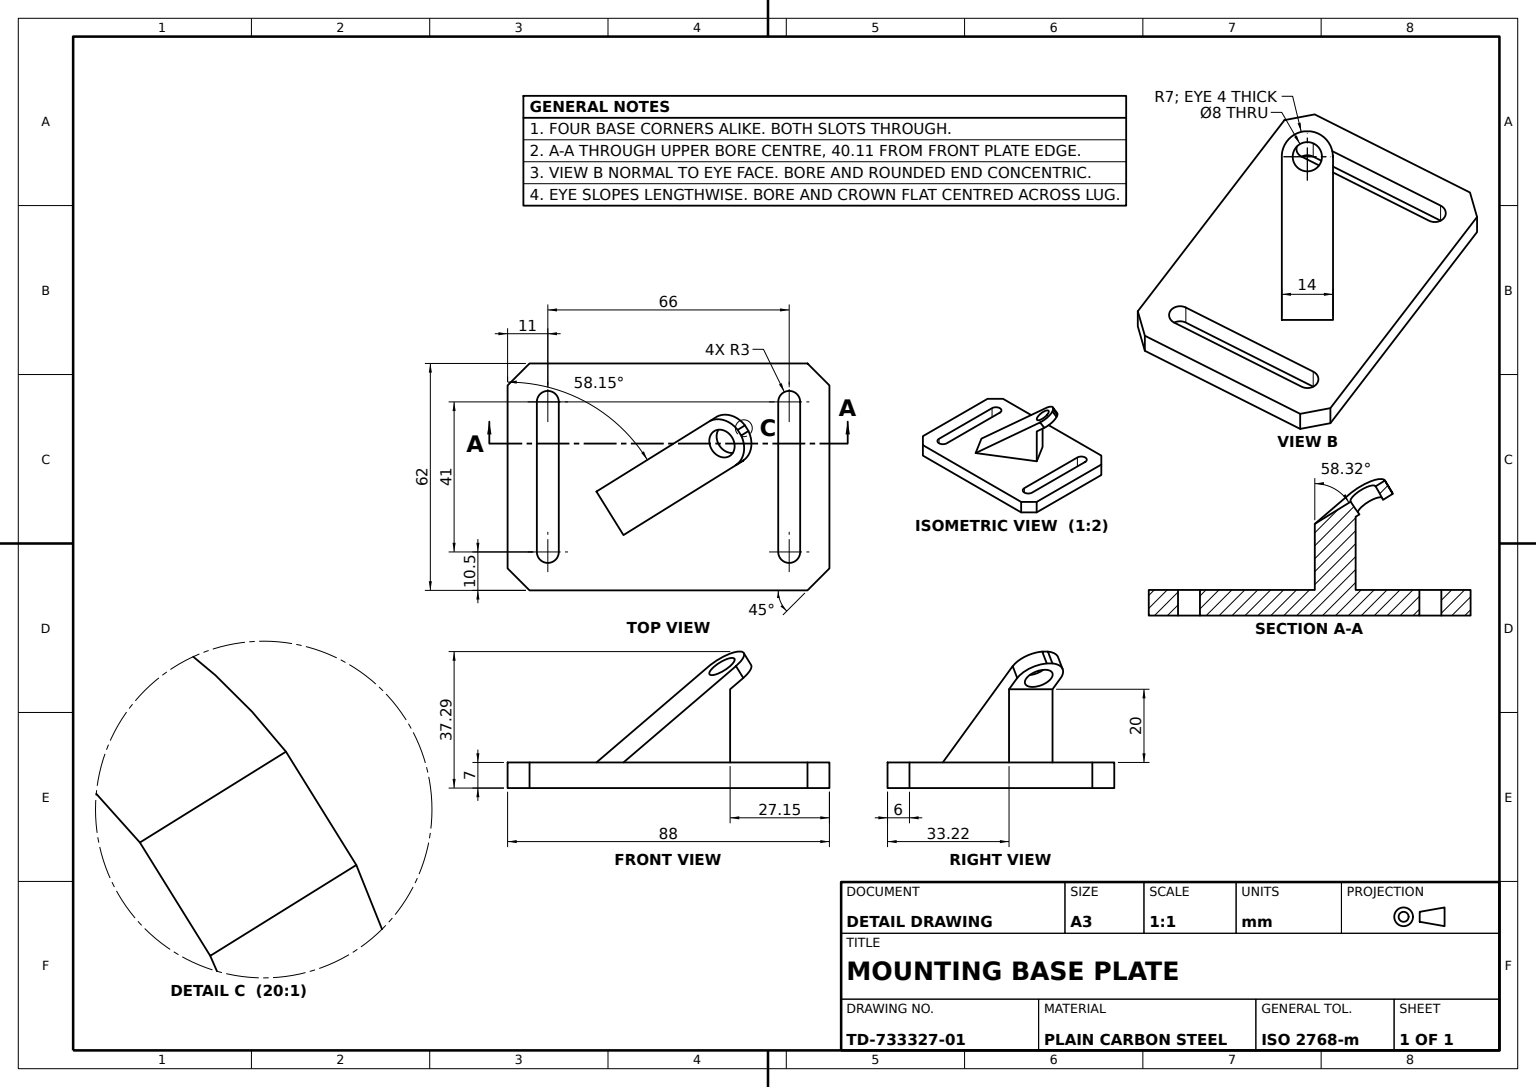
SolidWorks part; units mm, degrees
material "Plain Carbon Steel"
ref_plane "Front Plane" through (0, 0, 0) normal (0, 0, 1) x (1, 0, 0)
ref_plane "Top Plane" through (0, 0, 0) normal (0, 1, 0) x (1, 0, 0)
ref_plane "Right Plane" through (0, 0, 0) normal (1, 0, 0) x (0, 0, -1)
sketch "Base Plate Profile" plane through (0, 0, 0) normal (0, 1, 0) x (1, 0, 0)
  line L0 (-33, 20.5) -> (-33, -20.5) construction
  line L1 (-44, -31) -> (44, -31)
  line L2 (-44, -31) -> (-44, 31)
  line L3 (-44, 31) -> (44, 31)
  line L4 (44, -31) -> (44, 31)
  line L5 (-30, 20.5) -> (-30, -20.5)
  line L6 (-36, 20.5) -> (-36, -20.5)
  line L7 (33, 20.5) -> (33, -20.5) construction
  line L8 (36, 20.5) -> (36, -20.5)
  line L9 (30, 20.5) -> (30, -20.5)
  arc A0 (-30, 20.5) -> (-36, 20.5) centre (-33, 20.5) ccw
  arc A1 (-36, -20.5) -> (-30, -20.5) centre (-33, -20.5) ccw
  arc A2 (36, 20.5) -> (30, 20.5) centre (33, 20.5) ccw
  arc A3 (30, -20.5) -> (36, -20.5) centre (33, -20.5) ccw
  point P0 (0, 0)
  point P8 (-33, 0)
  point P13 (33, 0)
  dimension "D1" = 88
  dimension "D2" = 62
  dimension "D3" = 6
  dimension "D4" = 6
  dimension "D5" = 8
  dimension "D6" = 8
  dimension "D7" = 44
  dimension "D8" = 10.5
  dimension "D9" = 31
  dimension "D10" = 10.5
  dimension "D11" = 41
  dimension "D12" = 41
extrude "Base Plate 88x62x7" add sketch "Base Plate Profile" along normal blind 7
chamfer "Plate Edge Chamfer 6mm" distance 6 angle 45 4 edges at (-44, 3.5, -31) (44, 3.5, -31) (44, 3.5, 31) (-44, 3.5, 31)
sketch "Lug Profile" plane through (0, 7, 0) normal (0, 1, 0) x (1, 0, 0)
  line L0 (-19.705, -4.0002) -> (-12.3174, -15.8924)
  line L1 (-12.3174, -15.8924) -> (49.797, 22.6938)
  line L2 (49.797, 22.6938) -> (42.4094, 34.5859)
  line L3 (-55.7736, -34.6473) -> (54.8921, 34.0997) construction
  line L4 (42.4094, 34.5859) -> (-19.705, -4.0002)
  line L5 (-44, 25) -> (-44, -25) construction
  line L6 (38, 31) -> (-38, 31) construction
  dimension "D1" = 14
  dimension "D2" = 7
  dimension "D3" = 24.295
  dimension "D4" = 86.4094
  dimension "D5" = 31.6826
  dimension "D6" = 3.5859
extrude "Lifting Lug" add sketch "Lug Profile" along normal blind 87
sketch "Lug Taper Cut Profile" plane through (3.6938, 0, 5.9461) normal (0.5277, 0, 0.8494) x (0.8494, 0, -0.5277)
  line L0 (-18.8491, 7) -> (22.8408, 37.2895)
  line L1 (22.8408, 37.2895) -> (25.192, 34.0534)
  line L2 (25.192, 34.0534) -> (15.4838, 27)
  line L3 (15.4838, 27) -> (15.4838, 7)
  line L4 (24.1833, 7) -> (47.4503, 7) construction
  line L5 (-18.8491, 7) -> (-91.2168, 88.0489)
  line L6 (-91.2168, 88.0489) -> (-3.0961, 106.6936)
  line L15 (-3.0961, 106.6936) -> (102.8843, 93.1517)
  line L16 (102.8843, 93.1517) -> (104.4544, 45.6568)
  line L17 (104.4544, 45.6568) -> (67.8834, 13.003)
  line L18 (67.8834, 13.003) -> (61.1603, 7)
  line L19 (61.1603, 7) -> (15.4838, 7)
  line L20 (-18.8491, 7) -> (30.9688, 7) construction
  dimension "D1" = 20
  dimension "D2" = 4
  dimension "D3" = 6.8856
  dimension "D4" = 12
  dimension "D5" = 13.6087
  dimension "D6" = 48.6096
  dimension "D7" = 50.1797
  dimension "D8" = 29.0827
  dimension "D9" = 57.3708
  dimension "D10" = 145.4915
  dimension "D11" = 6.003
  dimension "D12" = 86.1517
  dimension "D13" = 99.6936
extrude "Lug Taper Cut" cut sketch "Lug Taper Cut Profile" against normal blind 87
sketch "Lug Trim Profile" plane through (-8.3593, 13.5448, 5.1929) normal (-0.4993, 0.809, 0.3102) x (0.8664, 0.4662, 0.1787)
  line L4 (21.786, 25.5542) -> (25.4127, 37.4189)
  line L5 (-13.0947, -1.2293) -> (27.7775, 30.1548) construction
  line L6 (25.4127, 37.4189) -> (44.8629, 15.6604)
  line L7 (44.8629, 15.6604) -> (35.1378, 16.9374)
  line L8 (35.1378, 16.9374) -> (30.8242, 14.8773)
  arc A0 (30.8242, 14.8773) -> (21.786, 25.5542) centre (26.5195, 20.3973) ccw
  dimension "D1" = 14
  dimension "D2" = 8.5589
  dimension "D3" = 1.1661
  dimension "D4" = 5.4797
  dimension "D5" = 9.7844
  dimension "D6" = 10.8912
  dimension "D7" = 14.5179
  dimension "D8" = 27.9938
  dimension "D9" = 29.2708
  dimension "D10" = 49.7523
extrude "Lug Trim Cut" cut sketch "Lug Trim Profile" against normal blind 7
sketch "Lug Eye Hole Profile" plane through (-8.3593, 13.5448, 5.1929) normal (-0.4993, 0.809, 0.3102) x (0.8664, 0.4662, 0.1787)
  circle A0 centre (26.5195, 20.3973) radius 4
  dimension "D1" = 8
extrude "Lug Eye Hole" cut sketch "Lug Eye Hole Profile" against normal blind 17
